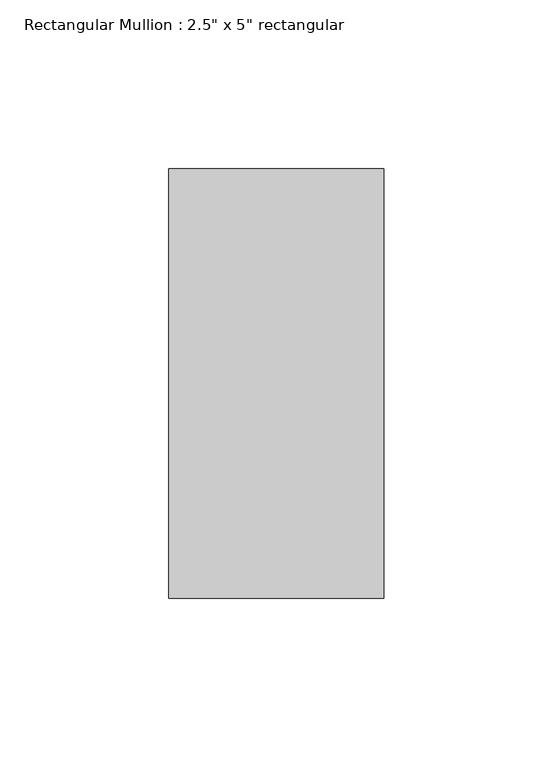
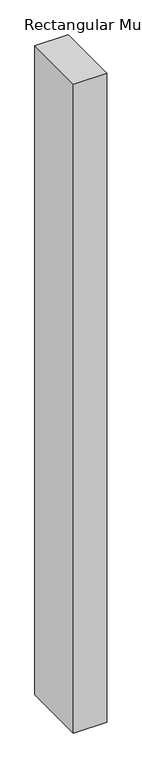
"""IFC4 building model written with IfcOpenShell, lengths in millimetres: member geometry."""

from ifc_helpers import new_model, si_unit, frame, origin, place, context, project, spatial, polyline, outline, extrude, source, transform, mapped, element, save


def member_d37749d9(model_context):
    return source(origin(), model_context, "Body", "SweptSolid", [
        extrude(outline(polyline([(0.0, 63.5), (0.0, -63.5), (-63.5, -63.5), (-63.5, 63.5), (0.0, 63.5)])), frame((0.0, 0.0, -1308.1), z_axis=(0.0, 0.0, 1.0), x_axis=(1.0, 0.0, 0.0)), (0.0, 0.0, 1.0), 1308.1),
    ])


if __name__ == "__main__":
    model = new_model("IFC4")
    model_context = context("Model", 3, world=origin())
    ifc_project = project(units=[si_unit("LENGTHUNIT", "METRE", prefix="MILLI")], contexts=[model_context])
    site = spatial("IfcSite", under=ifc_project)
    building = spatial("IfcBuilding", under=site)
    placement = place(None, origin())
    member_shape = member_d37749d9(model_context)
    element("IfcMember", 1, ObjectType="Rectangular Mullion : 2.5\" x 5\" rectangular", at=placement, inside=building, context=model_context, shape_type="MappedRepresentation", body=[
        mapped(member_shape, transform((0.0, 0.0, 0.0), x_axis=(1.0, 0.0, 0.0), y_axis=(0.0, 1.0, 0.0), z_axis=(0.0, 0.0, 1.0))),
    ])
    save(model, "model.ifc")

# Revit data of these elements
# Type "Rectangular Mullion : 2.5\" x 5\" rectangular"
#   built-in parameter 1007304 = 0.416667 (stored number, unit not read)
#   built-in parameter 1007301 = 0.104167 (stored number, unit not read)
#   built-in parameter 1007300 = 0.104167 (stored number, unit not read)
# Element 1 (IfcMember, "Rectangular Mullion : 2.5\" x 5\" rectangular")
#   Materials on its faces: "Aluminum"
# Materials
#   "Aluminum": class "Metal", colour RGB 247 247 247, transparency 0, Description = "Aluminum 6061", Cost = 0
